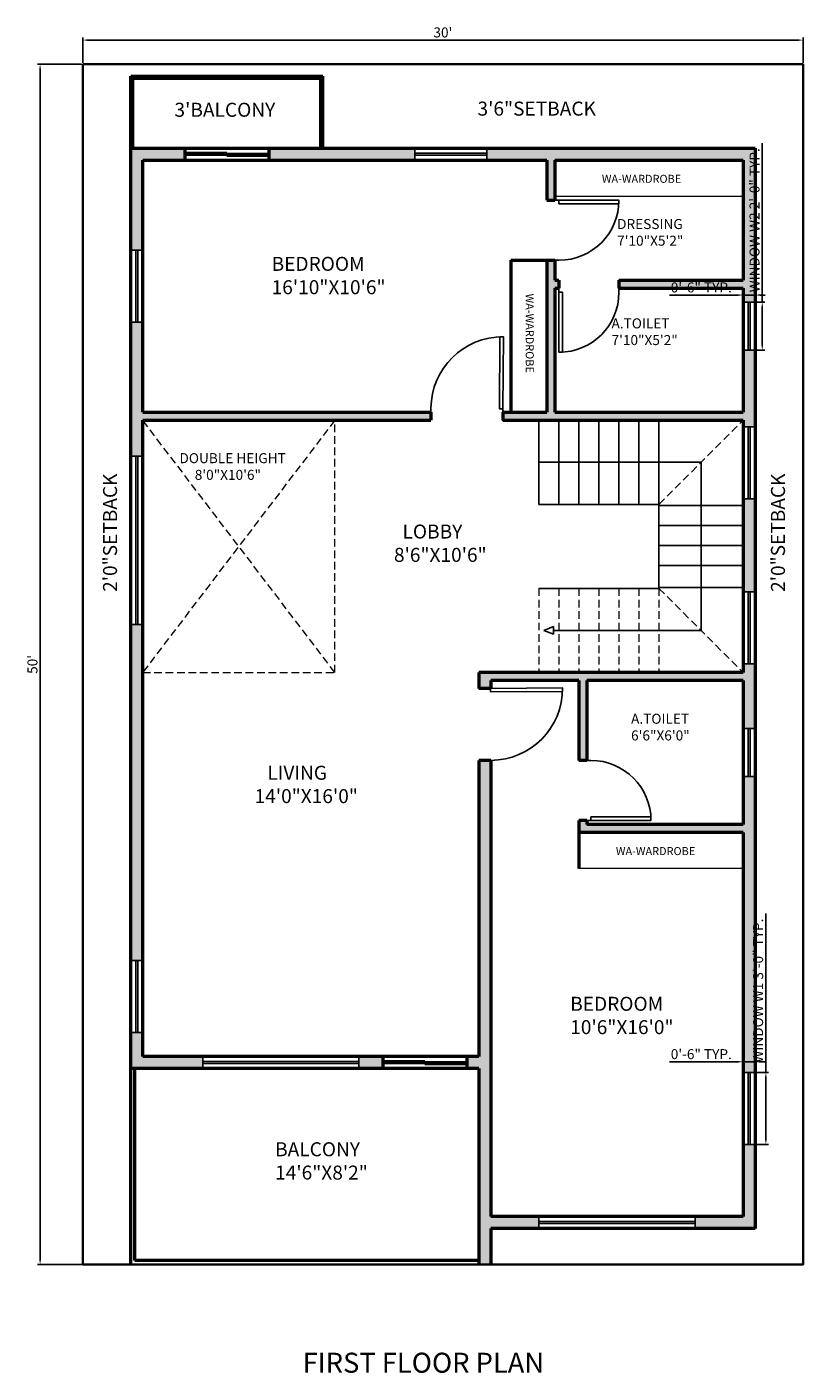
# Model space of a CAD drawing. Units: inches. Extents: x 2638 to 4577, y 1946 to 2619.
# Tile 8 of 8: x 4189 to 4577, y 1946 to 2619. Entities that reach past the tile are written whole.
import ezdxf

# ---------------------------------------------------------------- set-up
doc = ezdxf.new("R2010")
doc.units = ezdxf.units.IN
doc.linetypes.add('DASHED', pattern=[19.05, 12.7, -6.35])
for name, color, linetype, lineweight in [('A-ANNO-DIMS', 2, 'Continuous', 18), ('A-ANNO-TEXT', 7, 'Continuous', 25), ('A-AREA-IDEN', 7, 'Continuous', 25), ('A-DOOR', 4, 'Continuous', 25), ('A-FLOR-OVHD', 8, 'DASHED', 18), ('A-FLOR-STRS', 3, 'Continuous', 25), ('A-FURN', 8, 'Continuous', 18), ('A-GLAZ', 4, 'Continuous', 25), ('A-WALL', 7, 'Continuous', 50), ('A-WALL-PATT', 8, 'Continuous', 13), ('C-PROP', 1, 'Continuous', 35)]:
    doc.layers.add(name, color=color, linetype=linetype, lineweight=lineweight)
doc.styles.get("Standard").update_dxf_attribs({"font": 'arial.ttf'})
doc.dimstyles.new('ISO-25', dxfattribs={"dimtxt": 5, "dimasz": 2.5, "dimexe": 1.25, "dimexo": 0.625, "dimtad": 1, "dimdec": 1, "dimlunit": 3, "dimtxsty": 'Standard', "dimcen": 2.5, "dimclrt": 1, "dimadec": 0, "dimazin": 0, "dimtfac": 1, "dimtdec": 1, "dimtmove": 0, "dimatfit": 3, "dimfxl": 1, "dimarcsym": 0})

# ---------------------------------------------------------------- blocks, each defined once
blk = doc.blocks.new('*D37')
at = {"layer": 'A-ANNO-DIMS', "color": 0, "lineweight": -2, "transparency": 16777216}
for p, q in [((4216.58, 2600.78), (4216.58, 2613.44)), ((4219.08, 2612.19), (4574.08, 2612.19)), ((4576.58, 2600.78), (4576.58, 2613.44))]:
    blk.add_line(p, q, dxfattribs=at)
at = {"layer": 'A-ANNO-DIMS', "color": 0, "transparency": 16777216}
for points in [[(4219.08, 2612.61), (4219.08, 2611.77), (4216.58, 2612.19)], [(4574.08, 2612.61), (4574.08, 2611.77), (4576.58, 2612.19)]]:
    blk.add_solid(points, dxfattribs=at)
at = {"layer": 'Defpoints', "color": 0, "transparency": 16777216}
for p in [(4576.58, 2612.19), (4216.58, 2600.16), (4576.58, 2600.16)]:
    blk.add_point(p, dxfattribs=at)
at = {"layer": 'A-ANNO-DIMS', "color": 0, "transparency": 16777216, "insert": (4396.58, 2615.37), "char_height": 5, "attachment_point": 5}
blk.add_mtext("30'", dxfattribs=at)
blk = doc.blocks.new('*D38')
at = {"layer": 'A-ANNO-DIMS', "color": 0, "lineweight": -2, "transparency": 16777216}
for p, q in [((4215.96, 2600.16), (4194.04, 2600.16)), ((4195.29, 2597.66), (4195.29, 2002.66)), ((4215.96, 2000.16), (4194.04, 2000.16))]:
    blk.add_line(p, q, dxfattribs=at)
at = {"layer": 'A-ANNO-DIMS', "color": 0, "transparency": 16777216}
for points in [[(4194.87, 2597.66), (4195.7, 2597.66), (4195.29, 2600.16)], [(4194.87, 2002.66), (4195.7, 2002.66), (4195.29, 2000.16)]]:
    blk.add_solid(points, dxfattribs=at)
at = {"layer": 'Defpoints', "color": 0, "transparency": 16777216}
for p in [(4216.58, 2600.16), (4195.29, 2000.16), (4216.58, 2000.16)]:
    blk.add_point(p, dxfattribs=at)
at = {"layer": 'A-ANNO-DIMS', "color": 0, "transparency": 16777216, "insert": (4192.11, 2300.16), "char_height": 5, "attachment_point": 5, "rotation": 90}
blk.add_mtext("50'", dxfattribs=at)
blk = doc.blocks.new('*U5')
for p, q in [((0, 0), (0, -6)), ((30, 0), (30, -6))]:
    blk.add_line(p, q)
blk.add_lwpolyline([(0, 0), (0, 30), (1.75, 30), (1.75, 0)], close=True)
blk.add_arc((0, 0), 30, 0, 90)
blk = doc.blocks.new('*U4')
for p, q in [((0, 0), (0, -6)), ((36, 0), (36, -6))]:
    blk.add_line(p, q)
blk.add_lwpolyline([(0, 0), (0, 36), (1.75, 36), (1.75, 0)], close=True)
blk.add_arc((0, 0), 36, 0, 90)
blk = doc.blocks.new('WIN-36')
for p, q in [((2761.41, 2540.16), (2761.41, 2534.16)), ((2761.41, 2537.66), (2797.41, 2537.66)), ((2761.41, 2536.66), (2797.41, 2536.66)), ((2797.41, 2540.16), (2797.41, 2534.16))]:
    blk.add_line(p, q)
blk = doc.blocks.new('WIN-24')
for p, q in [((2905.41, 2558.16), (2905.41, 2552.16)), ((2929.41, 2558.16), (2929.41, 2552.16)), ((2905.41, 2555.66), (2929.41, 2555.66)), ((2905.41, 2554.66), (2929.41, 2554.66))]:
    blk.add_line(p, q)
blk = doc.blocks.new('WIN-84')
for p, q in [((2695.41, 2404.16), (2689.41, 2404.16)), ((2691.91, 2404.16), (2691.91, 2320.16)), ((2692.91, 2404.16), (2692.91, 2320.16)), ((2695.41, 2320.16), (2689.41, 2320.16))]:
    blk.add_line(p, q)
blk = doc.blocks.new('WIN-78')
for p, q in [((3314.99, 2024.16), (3314.99, 2018.16)), ((3314.99, 2021.66), (3392.99, 2021.66)), ((3314.99, 2020.66), (3392.99, 2020.66)), ((3392.99, 2024.16), (3392.99, 2018.16))]:
    blk.add_line(p, q)
blk = doc.blocks.new('*D47')
at = {"layer": 'A-ANNO-DIMS', "color": 0, "lineweight": -2, "transparency": 16777216}
for p, q in [((4557.98, 2096.16), (4557.98, 2175.6)), ((4553.21, 2096.16), (4559.23, 2096.16)), ((4557.98, 2062.66), (4557.98, 2093.66)), ((4553.21, 2060.16), (4559.23, 2060.16))]:
    blk.add_line(p, q, dxfattribs=at)
at = {"layer": 'A-ANNO-DIMS', "color": 0, "transparency": 16777216}
for points in [[(4557.57, 2093.66), (4558.4, 2093.66), (4557.98, 2096.16)], [(4557.57, 2062.66), (4558.4, 2062.66), (4557.98, 2060.16)]]:
    blk.add_solid(points, dxfattribs=at)
at = {"layer": 'Defpoints', "color": 0, "transparency": 16777216}
for p in [(4552.58, 2096.16), (4557.98, 2096.16), (4552.58, 2060.16)]:
    blk.add_point(p, dxfattribs=at)
at = {"layer": 'A-ANNO-DIMS', "color": 1, "transparency": 16777216, "insert": (4554.77, 2137.13), "char_height": 5, "attachment_point": 5, "rotation": 90}
blk.add_mtext('WINDOW W1 3\'-0" TYP.', dxfattribs=at)
blk = doc.blocks.new('*D48')
at = {"layer": 'A-ANNO-DIMS', "color": 0, "lineweight": -2, "transparency": 16777216}
for p, q in [((4544.08, 2101.56), (4509.86, 2101.56)), ((4546.58, 2096.78), (4546.58, 2102.81)), ((4552.58, 2101.56), (4546.58, 2101.56)), ((4552.58, 2096.78), (4552.58, 2102.81)), ((4555.08, 2101.56), (4557.58, 2101.56))]:
    blk.add_line(p, q, dxfattribs=at)
at = {"layer": 'A-ANNO-DIMS', "color": 0, "transparency": 16777216}
for points in [[(4544.08, 2101.97), (4544.08, 2101.14), (4546.58, 2101.56)], [(4555.08, 2101.97), (4555.08, 2101.14), (4552.58, 2101.56)]]:
    blk.add_solid(points, dxfattribs=at)
at = {"layer": 'Defpoints', "color": 0, "transparency": 16777216}
for p in [(4546.58, 2101.56), (4546.58, 2096.16), (4552.58, 2096.16)]:
    blk.add_point(p, dxfattribs=at)
at = {"layer": 'A-ANNO-DIMS', "color": 1, "transparency": 16777216, "insert": (4525.72, 2104.73), "char_height": 5, "attachment_point": 5}
blk.add_mtext('0\'-6" TYP.', dxfattribs=at)
blk = doc.blocks.new('*D49')
at = {"layer": 'A-ANNO-DIMS', "color": 0, "lineweight": -2, "transparency": 16777216}
for p, q in [((4556.18, 2481.16), (4556.18, 2560.6)), ((4553.21, 2481.16), (4557.43, 2481.16)), ((4556.18, 2459.66), (4556.18, 2478.66)), ((4553.21, 2457.16), (4557.43, 2457.16))]:
    blk.add_line(p, q, dxfattribs=at)
at = {"layer": 'A-ANNO-DIMS', "color": 0, "transparency": 16777216}
for points in [[(4555.77, 2478.66), (4556.6, 2478.66), (4556.18, 2481.16)], [(4555.77, 2459.66), (4556.6, 2459.66), (4556.18, 2457.16)]]:
    blk.add_solid(points, dxfattribs=at)
at = {"layer": 'Defpoints', "color": 0, "transparency": 16777216}
for p in [(4552.58, 2481.16), (4556.18, 2481.16), (4552.58, 2457.16)]:
    blk.add_point(p, dxfattribs=at)
at = {"layer": 'A-ANNO-DIMS', "color": 1, "transparency": 16777216, "insert": (4552.97, 2522.13), "char_height": 5, "attachment_point": 5, "rotation": 90}
blk.add_mtext('WINDOW W2 2\'-0" TYP.', dxfattribs=at)
blk = doc.blocks.new('*D50')
at = {"layer": 'A-ANNO-DIMS', "color": 0, "lineweight": -2, "transparency": 16777216}
for p, q in [((4544.08, 2484.76), (4509.86, 2484.76)), ((4546.58, 2481.78), (4546.58, 2486.01)), ((4552.58, 2484.76), (4546.58, 2484.76)), ((4552.58, 2481.78), (4552.58, 2486.01)), ((4555.08, 2484.76), (4557.58, 2484.76))]:
    blk.add_line(p, q, dxfattribs=at)
at = {"layer": 'A-ANNO-DIMS', "color": 0, "transparency": 16777216}
for points in [[(4544.08, 2485.17), (4544.08, 2484.34), (4546.58, 2484.76)], [(4555.08, 2485.17), (4555.08, 2484.34), (4552.58, 2484.76)]]:
    blk.add_solid(points, dxfattribs=at)
at = {"layer": 'Defpoints', "color": 0, "transparency": 16777216}
for p in [(4546.58, 2484.76), (4546.58, 2481.16), (4552.58, 2481.16)]:
    blk.add_point(p, dxfattribs=at)
at = {"layer": 'A-ANNO-DIMS', "color": 1, "transparency": 16777216, "insert": (4525.72, 2487.93), "char_height": 5, "attachment_point": 5}
blk.add_mtext('0\'-6" TYP.', dxfattribs=at)

msp = doc.modelspace()

# ---------------------------------------------------------------- hatches: boundary and pattern name
at = {"layer": 'A-WALL-PATT', "transparency": 33554687}
h = msp.add_hatch(color=256, dxfattribs=at)
h.dxf.hatch_style = 1
h.paths.add_polyline_path([(4246.58, 2552.16), (4267.58, 2552.16), (4267.58, 2558.16), (4240.58, 2558.16), (4240.58, 2507.16), (4246.58, 2507.16)])
h.paths.add_polyline_path([(4382.54, 2558.16), (4309.58, 2558.16), (4309.58, 2552.16), (4324, 2552.16), (4382.54, 2552.16)])
h.paths.add_polyline_path([(4552.58, 2558.16), (4418.54, 2558.16), (4418.54, 2552.16), (4448.58, 2552.16), (4448.58, 2532.16), (4452.58, 2532.16), (4452.58, 2552.16), (4546.58, 2552.16), (4546.58, 2492.16), (4484.58, 2492.16), (4484.58, 2488.16), (4546.58, 2488.16), (4546.58, 2481.16), (4552.58, 2481.16)])
h.paths.add_polyline_path([(4552.58, 2457.16), (4546.58, 2457.16), (4546.58, 2426.16), (4501.85, 2426.16), (4452.58, 2426.16), (4452.58, 2439.06), (4452.58, 2488.16), (4454.58, 2488.16), (4454.58, 2492.16), (4452.58, 2492.16), (4452.58, 2502.16), (4448.58, 2502.16), (4448.58, 2426.16), (4426.61, 2426.16), (4426.58, 2422.16), (4546.58, 2422.16), (4546.58, 2418.91), (4552.58, 2418.91)])
h.paths.add_polyline_path([(4276.58, 2104.16), (4246.58, 2104.16), (4246.58, 2116.16), (4240.58, 2116.16), (4240.58, 2098.16), (4276.58, 2098.16)])
h.paths.add_polyline_path([(4366.58, 2104.16), (4354.58, 2104.16), (4354.58, 2098.16), (4366.58, 2098.16)])
h.paths.add_polyline_path([(4420.58, 2252.16), (4414.58, 2252.16), (4414.58, 2104.16), (4408.58, 2104.16), (4408.58, 2098.16), (4414.58, 2098.16), (4414.58, 2000.16), (4420.58, 2000.16), (4420.58, 2018.16), (4444.58, 2018.16), (4444.58, 2024.16), (4420.58, 2024.16)])
h.paths.add_polyline_path([(4552.58, 2060.16), (4546.58, 2060.16), (4546.58, 2024.16), (4522.58, 2024.16), (4522.58, 2018.16), (4552.58, 2018.16)])
h.paths.add_polyline_path([(4552.58, 2244.16), (4546.58, 2244.16), (4546.58, 2220.16), (4501.85, 2220.16), (4468.58, 2220.16), (4468.58, 2222.16), (4464.58, 2222.16), (4464.58, 2216.16), (4546.58, 2216.16), (4546.58, 2096.16), (4552.58, 2096.16)])
h.paths.add_polyline_path([(4552.58, 2300.41), (4546.58, 2300.41), (4546.58, 2296.16), (4414.58, 2296.16), (4414.58, 2288.16), (4420.58, 2288.16), (4420.58, 2292.16), (4464.58, 2292.16), (4464.58, 2252.16), (4468.58, 2252.16), (4468.58, 2292.16), (4546.58, 2292.16), (4546.58, 2268.16), (4552.58, 2268.16)])
h.paths.add_polyline_path([(4552.58, 2382.91), (4546.58, 2382.91), (4546.58, 2336.41), (4552.58, 2336.41)])
h.paths.add_polyline_path([(4390.58, 2426.16), (4246.58, 2426.16), (4246.58, 2471.16), (4240.58, 2471.16), (4240.58, 2404.16), (4246.58, 2404.16), (4246.58, 2422.16), (4390.58, 2422.16)])
h.paths.add_polyline_path([(4246.58, 2320.16), (4240.58, 2320.16), (4240.58, 2152.16), (4246.58, 2152.16)])
h.paths.add_polyline_path([(4322.52, 2481.2), (4381.82, 2481.2), (4381.82, 2507.82), (4322.52, 2507.82)], flags=9)
h.paths.add_polyline_path([(4481.97, 2202.6), (4527.74, 2202.6), (4527.74, 2210.84), (4481.97, 2210.84)], flags=25)
h.paths.add_polyline_path([(4237.73, 2334.43), (4237.73, 2401.53), (4222.78, 2401.53), (4222.78, 2334.43)], flags=9)
h.paths.add_polyline_path([(4571.53, 2334.43), (4571.53, 2401.53), (4556.59, 2401.53), (4556.59, 2334.43)], flags=9)
h.paths.add_polyline_path([(4411.71, 2570.46), (4478.81, 2570.46), (4478.81, 2585.4), (4411.71, 2585.4)], flags=9)
h.paths.add_polyline_path([(4369.74, 2347.41), (4418.71, 2347.41), (4418.71, 2374.03), (4369.74, 2374.03)], flags=9)
h.paths.add_polyline_path([(4299.5, 2226.85), (4353.64, 2226.85), (4353.64, 2253.46), (4299.5, 2253.46)], flags=9)
h.paths.add_polyline_path([(4338.99, 2038.68), (4393.49, 2038.68), (4393.49, 2065.29), (4338.99, 2065.29)], flags=9)
h.paths.add_polyline_path([(4442.64, 2123.44), (4498.87, 2123.44), (4498.87, 2150.05), (4442.64, 2150.05)], flags=9)
h.paths.add_polyline_path([(4489.06, 2259.32), (4524.82, 2259.32), (4524.82, 2278.33), (4489.06, 2278.33)], flags=25)

# ---------------------------------------------------------------- linework, layer by layer
at = {"layer": 'A-FLOR-OVHD', "ltscale": 0.3}
for p, q in [((4342.58, 2296.16), (4246.58, 2422.16)), ((4342.58, 2422.16), (4246.58, 2296.16)), ((4342.58, 2296.16), (4342.58, 2422.16)), ((4504.58, 2380.16), (4546.58, 2422.16)), ((4444.58, 2338.16), (4444.58, 2296.16)), ((4454.58, 2338.16), (4454.58, 2296.16)), ((4464.58, 2338.16), (4464.58, 2296.16)), ((4474.58, 2338.16), (4474.58, 2296.16)), ((4484.58, 2338.16), (4484.58, 2296.16)), ((4494.58, 2338.16), (4494.58, 2296.16)), ((4504.58, 2338.16), (4504.58, 2296.16)), ((4504.58, 2338.16), (4546.58, 2296.16)), ((4246.58, 2296.16), (4342.58, 2296.16))]:
    msp.add_line(p, q, dxfattribs=at)
at = {"layer": 'A-FLOR-STRS'}
for p, q in [((4444.58, 2422.16), (4444.58, 2380.16)), ((4454.58, 2422.16), (4454.58, 2380.16)), ((4464.58, 2422.16), (4464.58, 2380.16)), ((4474.58, 2422.16), (4474.58, 2380.16)), ((4484.58, 2422.16), (4484.58, 2380.16)), ((4494.58, 2422.16), (4494.58, 2380.16)), ((4504.58, 2422.16), (4504.58, 2338.16)), ((4444.58, 2380.16), (4504.58, 2380.16)), ((4504.58, 2379.66), (4546.58, 2379.66)), ((4504.58, 2369.66), (4546.58, 2369.66)), ((4504.58, 2359.66), (4546.58, 2359.66)), ((4504.58, 2349.66), (4546.58, 2349.66)), ((4504.58, 2338.16), (4444.58, 2338.16)), ((4546.58, 2338.66), (4504.58, 2338.66))]:
    msp.add_line(p, q, dxfattribs=at)
msp.add_lwpolyline([(4444.58, 2401.16), (4525.58, 2401.16), (4525.58, 2317.16), (4451.81, 2317.16)], dxfattribs=at)
msp.add_lwpolyline([(4447.04, 2317.16), (4451.81, 2315.29), (4451.81, 2319.03)], close=True, dxfattribs=at)
at = {"layer": 'A-FURN'}
for p, q in [((4452.58, 2534.16), (4546.58, 2534.16)), ((4546.58, 2198.16), (4464.58, 2198.16))]:
    msp.add_line(p, q, dxfattribs=at)
at = {"layer": 'A-WALL'}
for p, q in [((4240.58, 2000.16), (4240.58, 2594.16)), ((4240.58, 2594.16), (4336.58, 2594.16)), ((4241.58, 2593.16), (4335.58, 2593.16)), ((4241.58, 2558.16), (4241.58, 2593.16)), ((4335.58, 2558.16), (4335.58, 2593.16)), ((4336.58, 2558.16), (4336.58, 2594.16)), ((4240.58, 2558.16), (4552.58, 2558.16)), ((4267.58, 2558.16), (4267.58, 2552.16)), ((4309.58, 2558.16), (4309.58, 2552.16)), ((4552.58, 2558.16), (4552.58, 2018.16)), ((4246.58, 2552.16), (4448.58, 2552.16)), ((4246.58, 2426.16), (4246.58, 2552.16)), ((4267.58, 2555.66), (4288.58, 2555.66)), ((4267.58, 2555.16), (4309.58, 2555.16)), ((4288.58, 2555.66), (4288.58, 2554.66)), ((4288.58, 2554.66), (4309.58, 2554.66)), ((4448.58, 2552.16), (4448.58, 2532.16)), ((4452.58, 2552.16), (4546.58, 2552.16)), ((4452.58, 2552.16), (4452.58, 2532.16)), ((4546.58, 2552.16), (4546.58, 2492.16)), ((4448.58, 2532.16), (4452.58, 2532.16)), ((4430.58, 2502.16), (4452.58, 2502.16)), ((4430.58, 2502.16), (4430.58, 2426.16)), ((4448.58, 2502.16), (4448.58, 2426.16)), ((4452.58, 2502.16), (4452.58, 2492.16)), ((4452.58, 2492.16), (4454.58, 2492.16)), ((4454.58, 2492.16), (4454.58, 2488.16)), ((4484.58, 2492.16), (4546.58, 2492.16)), ((4484.58, 2492.16), (4484.58, 2488.16)), ((4452.58, 2488.16), (4454.58, 2488.16)), ((4452.58, 2488.16), (4452.58, 2426.16)), ((4484.58, 2488.16), (4546.58, 2488.16)), ((4546.58, 2488.16), (4546.58, 2426.16)), ((4246.58, 2426.16), (4390.58, 2426.16)), ((4246.58, 2422.16), (4390.58, 2422.16)), ((4246.58, 2104.16), (4246.58, 2422.16)), ((4390.58, 2426.16), (4390.58, 2422.16)), ((4426.58, 2426.16), (4448.58, 2426.16)), ((4426.58, 2426.16), (4426.58, 2422.16)), ((4426.58, 2422.16), (4546.58, 2422.16)), ((4452.58, 2426.16), (4546.58, 2426.16)), ((4546.58, 2422.16), (4546.58, 2296.16)), ((4414.58, 2296.16), (4414.58, 2288.16)), ((4546.58, 2296.16), (4414.58, 2296.16)), ((4420.58, 2288.16), (4414.58, 2288.16)), ((4420.58, 2292.16), (4420.58, 2288.16)), ((4464.58, 2292.16), (4420.58, 2292.16)), ((4464.58, 2292.16), (4464.58, 2252.16)), ((4546.58, 2292.16), (4468.58, 2292.16)), ((4468.58, 2292.16), (4468.58, 2252.16)), ((4546.58, 2292.16), (4546.58, 2220.16)), ((4414.58, 2252.16), (4414.58, 2104.16)), ((4420.58, 2252.16), (4414.58, 2252.16)), ((4420.58, 2252.16), (4420.58, 2024.16)), ((4468.58, 2252.16), (4464.58, 2252.16)), ((4464.58, 2222.16), (4464.58, 2198.16)), ((4468.58, 2222.16), (4464.58, 2222.16)), ((4468.58, 2222.16), (4468.58, 2220.16)), ((4546.58, 2216.16), (4464.58, 2216.16)), ((4546.58, 2220.16), (4468.58, 2220.16)), ((4546.58, 2216.16), (4546.58, 2024.16)), ((4414.58, 2104.16), (4246.58, 2104.16)), ((4366.58, 2104.16), (4366.58, 2098.16)), ((4366.58, 2101.66), (4387.58, 2101.66)), ((4366.58, 2101.16), (4408.58, 2101.16)), ((4387.58, 2101.66), (4387.58, 2100.66)), ((4387.58, 2100.66), (4408.58, 2100.66)), ((4408.58, 2104.16), (4408.58, 2098.16)), ((4414.58, 2098.16), (4240.58, 2098.16)), ((4242.58, 2002.16), (4242.58, 2098.16)), ((4414.58, 2098.16), (4414.58, 2000.16)), ((4546.58, 2024.16), (4420.58, 2024.16)), ((4420.58, 2018.16), (4420.58, 2000.16)), ((4552.58, 2018.16), (4420.58, 2018.16)), ((4414.58, 2002.16), (4242.58, 2002.16))]:
    msp.add_line(p, q, dxfattribs=at)
at = {"layer": 'C-PROP'}
msp.add_line((4216.58, 2207.16), (4216.58, 2290.16), dxfattribs=at)
msp.add_lwpolyline([(4216.58, 2600.16), (4576.58, 2600.16), (4576.58, 2000.16), (4216.58, 2000.16)], close=True, dxfattribs=at)

# ---------------------------------------------------------------- block references
at = {"layer": 'A-DOOR'}
for name, p, rotation in [('*U5', (4454.58, 2532.16), 270), ('*U4', (4420.38, 2288.19), 270.3213350750104)]:
    msp.add_blockref(name, p, dxfattribs=dict(at, rotation=rotation))
at = {"layer": 'A-DOOR', "xscale": -1}
for name, p, rotation in [('*U5', (4454.58, 2486.16), 180), ('*U4', (4426.62, 2427.95), 359.6786649249896), ('*U5', (4470.58, 2222.16), 270)]:
    msp.add_blockref(name, p, dxfattribs=dict(at, rotation=rotation))
at = {"layer": 'A-GLAZ'}
for name, p in [('WIN-36', (1621.13, 18)), ('WIN-84', (1551.17, 0))]:
    msp.add_blockref(name, p, dxfattribs=at)
for name, p, rotation in [('WIN-36', (1706.43, 5268.57), 270), ('WIN-24', (7104.74, -448.25), 90.00000000001023), ('WIN-36', (2012.43, 5180.32), 270.0000000000059), ('WIN-36', (7086.74, -461), 90.00000000000254), ('WIN-24', (7104.74, -661.25), 90.00000000001074), ('WIN-36', (6780.74, -645.25), 90.00000000000585), ('WIN-78', (7669.57, 4122.31), 180), ('WIN-36', (7086.74, -701.25), 90.00000000000561), ('WIN-78', (7837.57, 4042.31), 180)]:
    msp.add_blockref(name, p, dxfattribs=dict(at, rotation=rotation))

# ---------------------------------------------------------------- texts
at = {"layer": 'A-ANNO-TEXT', "attachment_point": 1}
for s, width, insert, char_height in [("{\\fTimes New Roman|b0|i0|c0|p18;3'BALCONY}", 61.0557, (4262.44, 2580.87), 7), ('{\\fTimes New Roman|b0|i0|c0|p18;3\'6"SETBACK}', 61.0557, (4413.88, 2581.44), 7), ('WA-WARDROBE', 29.5334, (4476.03, 2544.86), 4), ('WA-WARDROBE', 29.5334, (4483.04, 2208.86), 4), ('{\\fTimes New Roman|b0|i0|c0|p18;FIRST FLOOR PLAN}', 196.2607, (4326.5, 1956.14), 10)]:
    msp.add_mtext_dynamic_manual_height_columns(s, width=width, gutter_width=12.5, heights=[0], dxfattribs=dict(at, insert=insert, char_height=char_height))
for s, width, insert, char_height, rotation in [('WA-WARDROBE', 29.5334, (4441.99, 2485.51), 4, 270), ('{\\fTimes New Roman|b0|i0|c0|p18;2\'0"SETBACK}', 61.0557, (4226.74, 2336.4), 7, 90), ('{\\fTimes New Roman|b0|i0|c0|p18;2\'0"SETBACK}', 61.0557, (4560.55, 2336.4), 7, 90)]:
    msp.add_mtext_dynamic_manual_height_columns(s, width=width, gutter_width=12.5, heights=[0], dxfattribs=dict(at, insert=insert, char_height=char_height, rotation=rotation))
at = {"layer": 'A-AREA-IDEN', "attachment_point": 1}
for s, width, insert, char_height in [('{\\fTimes New Roman|b0|i0|c0|p18;DRESSING\\P7\'10"X5\'2"}', 61.0557, (4483.65, 2522.76), 5), ('{\\fTimes New Roman|b0|i0|c0|p18;BEDROOM\\P16\'10"X10\'6"}', 61.0557, (4310.99, 2503.86), 7), ('{\\fTimes New Roman|b0|i0|c0|p18;A.TOILET\\P7\'10"X5\'2"}', 61.0557, (4480.86, 2473.1), 5), ('{\\fTimes New Roman|b0|i0|c0|p18;DOUBLE HEIGHT\\P     8\'0"X10\'6"}', 88.9051, (4264.94, 2405.74), 5), ('{\\fTimes New Roman|b0|i0|c0|p18;  LOBBY\\P8\'6"X10\'6"}', 61.0557, (4372.12, 2370.07), 7), ('{\\fTimes New Roman|b0|i0|c0|p18;A.TOILET\\P6\'6"X6\'0"}', 61.0557, (4490.62, 2275.5), 5), ('{\\fTimes New Roman|b0|i0|c0|p18;   LIVING\\P14\'0"X16\'0"}', 61.0557, (4302.47, 2249.5), 7), ('{\\fTimes New Roman|b0|i0|c0|p18;BEDROOM\\P10\'6"X16\'0"}', 61.0557, (4460.21, 2134.03), 7), ('{\\fTimes New Roman|b0|i0|c0|p18;BALCONY\\P14\'6"X8\'2"}', 61.0557, (4312.73, 2061.33), 7)]:
    msp.add_mtext_dynamic_manual_height_columns(s, width=width, gutter_width=12.5, heights=[0], dxfattribs=dict(at, insert=insert, char_height=char_height))

# ---------------------------------------------------------------- dimensions: what is measured, and where the dimension line sits
at = {"layer": 'A-ANNO-DIMS'}
dim = msp.add_linear_dim(base=(4576.58, 2612.19), p1=(4216.58, 2600.16), p2=(4576.58, 2600.16), dimstyle='ISO-25', override={"dimclrd": 0, "dimclre": 0, "dimclrt": 0}, dxfattribs=at)
dim.commit()
dim.dimension.update_dxf_attribs({"geometry": '*D37', "text_midpoint": (4396.58, 2615.37)})
dim = msp.add_linear_dim(base=(4195.29, 2000.16), p1=(4216.58, 2600.16), p2=(4216.58, 2000.16), angle=90, dimstyle='ISO-25', override={"dimclrd": 0, "dimclre": 0, "dimclrt": 0}, dxfattribs=at)
dim.commit()
dim.dimension.update_dxf_attribs({"geometry": '*D38', "text_midpoint": (4192.11, 2300.16)})
for base, p1, p2, angle, text, picture, middle in [((4556.18, 2481.16), (4552.58, 2457.16), (4552.58, 2481.16), 90, 'WINDOW W2 <> TYP.', '*D49', (4552.97, 2522.13)), ((4546.58, 2484.76), (4552.58, 2481.16), (4546.58, 2481.16), 180, '<> TYP.', '*D50', (4525.72, 2487.93)), ((4557.98, 2096.16), (4552.58, 2060.16), (4552.58, 2096.16), 90, 'WINDOW W1 <> TYP.', '*D47', (4554.77, 2137.13)), ((4546.58, 2101.56), (4552.58, 2096.16), (4546.58, 2096.16), 180, '<> TYP.', '*D48', (4525.72, 2104.73))]:
    dim = msp.add_linear_dim(base=base, p1=p1, p2=p2, angle=angle, text=text, dimstyle='ISO-25', override={"dimdec": 1, "dimrnd": 0, "dimzin": 1, "dimlunit": 4, "dimfrac": 2}, dxfattribs=at)
    dim.commit()
    dim.dimension.update_dxf_attribs({"geometry": picture, "text_midpoint": middle})

doc.saveas('drawing.dxf')
